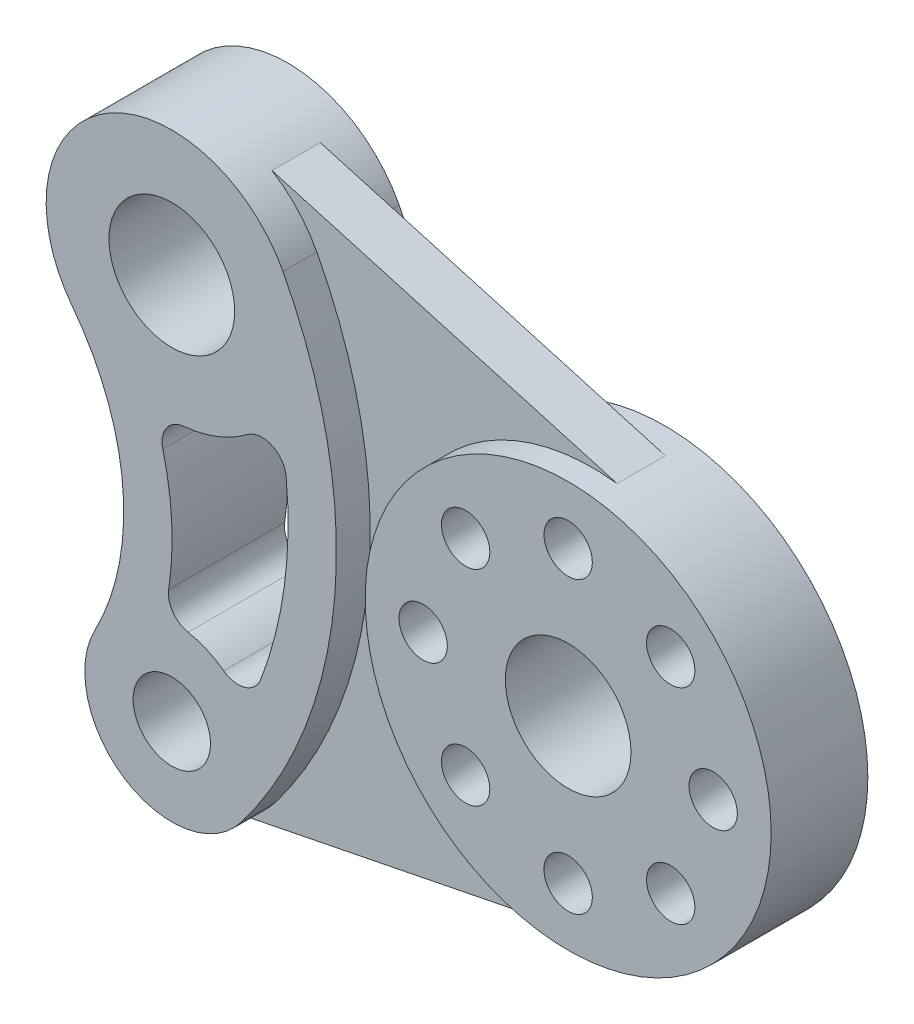
ISO-10303-21;
HEADER;
FILE_DESCRIPTION(('STEP AP214'),'2;1');
FILE_NAME('part.step','',(''),(''),'','','');
FILE_SCHEMA(('AUTOMOTIVE_DESIGN { 1 0 10303 214 1 1 1 1 }'));
ENDSEC;
DATA;
#1=APPLICATION_CONTEXT('core data for automotive mechanical design processes');
#2=APPLICATION_PROTOCOL_DEFINITION('international standard','automotive_design',2000,#1);
#3=PRODUCT_CONTEXT('',#1,'mechanical');
#4=PRODUCT('Part','Part','',(#3));
#5=PRODUCT_RELATED_PRODUCT_CATEGORY('part','',(#4));
#6=PRODUCT_DEFINITION_FORMATION('','',#4);
#7=PRODUCT_DEFINITION_CONTEXT('part definition',#1,'design');
#8=PRODUCT_DEFINITION('design','',#6,#7);
#9=PRODUCT_DEFINITION_SHAPE('','',#8);
#10=(LENGTH_UNIT() NAMED_UNIT(*) SI_UNIT(.MILLI.,.METRE.));
#11=(NAMED_UNIT(*) PLANE_ANGLE_UNIT() SI_UNIT($,.RADIAN.));
#12=(NAMED_UNIT(*) SI_UNIT($,.STERADIAN.) SOLID_ANGLE_UNIT());
#13=UNCERTAINTY_MEASURE_WITH_UNIT(LENGTH_MEASURE(1.E-05),#10,'distance_accuracy_value','');
#14=(GEOMETRIC_REPRESENTATION_CONTEXT(3) GLOBAL_UNCERTAINTY_ASSIGNED_CONTEXT((#13)) GLOBAL_UNIT_ASSIGNED_CONTEXT((#10,
#11,#12)) REPRESENTATION_CONTEXT('',''));
#15=CARTESIAN_POINT('',(0.,0.,0.));
#16=DIRECTION('',(0.,0.,1.));
#17=DIRECTION('',(1.,0.,0.));
#18=AXIS2_PLACEMENT_3D('',#15,#16,#17);
#19=CARTESIAN_POINT('',(-80.,-40.,24.));
#20=DIRECTION('',(0.,0.,-1.));
#21=DIRECTION('',(-1.,0.,0.));
#22=AXIS2_PLACEMENT_3D('',#19,#20,#21);
#23=CYLINDRICAL_SURFACE('',#22,18.);
#24=CARTESIAN_POINT('',(-80.,-40.,17.));
#25=DIRECTION('',(0.,0.,-1.));
#26=DIRECTION('',(-1.,0.,0.));
#27=AXIS2_PLACEMENT_3D('',#24,#25,#26);
#28=CIRCLE('',#27,18.);
#29=CARTESIAN_POINT('',(-65.7048938733706,-50.9384615384615,17.));
#30=VERTEX_POINT('',#29);
#31=CARTESIAN_POINT('',(-73.0769230769233,-56.6153846153847,17.));
#32=VERTEX_POINT('',#31);
#33=EDGE_CURVE('E230',#30,#32,#28,.T.);
#34=ORIENTED_EDGE('',*,*,#33,.F.);
#35=DIRECTION('',(0.,0.,-1.));
#36=VECTOR('',#35,1.);
#37=CARTESIAN_POINT('',(-65.7048938733706,-50.9384615384615,24.));
#38=LINE('',#37,#36);
#39=CARTESIAN_POINT('',(-65.7048938733706,-50.9384615384615,24.));
#40=VERTEX_POINT('',#39);
#41=EDGE_CURVE('E326',#40,#30,#38,.T.);
#42=ORIENTED_EDGE('',*,*,#41,.F.);
#43=CARTESIAN_POINT('',(-80.,-40.,24.));
#44=DIRECTION('',(0.,0.,1.));
#45=DIRECTION('',(1.,0.,0.));
#46=AXIS2_PLACEMENT_3D('',#43,#44,#45);
#47=CIRCLE('',#46,18.);
#48=CARTESIAN_POINT('',(-95.9288325411013,-31.6171428571429,24.));
#49=VERTEX_POINT('',#48);
#50=EDGE_CURVE('E271',#49,#40,#47,.T.);
#51=ORIENTED_EDGE('',*,*,#50,.F.);
#52=DIRECTION('',(0.,0.,-1.));
#53=VECTOR('',#52,1.);
#54=CARTESIAN_POINT('',(-95.9288325411013,-31.6171428571429,24.));
#55=LINE('',#54,#53);
#56=CARTESIAN_POINT('',(-95.9288325411013,-31.6171428571429,0.));
#57=VERTEX_POINT('',#56);
#58=EDGE_CURVE('E335',#49,#57,#55,.T.);
#59=ORIENTED_EDGE('',*,*,#58,.T.);
#60=CARTESIAN_POINT('',(-80.,-40.,0.));
#61=DIRECTION('',(0.,0.,1.));
#62=DIRECTION('',(1.,0.,0.));
#63=AXIS2_PLACEMENT_3D('',#60,#61,#62);
#64=CIRCLE('',#63,18.);
#65=CARTESIAN_POINT('',(-65.7048938733706,-50.9384615384615,0.));
#66=VERTEX_POINT('',#65);
#67=EDGE_CURVE('E312',#57,#66,#64,.T.);
#68=ORIENTED_EDGE('',*,*,#67,.T.);
#69=CARTESIAN_POINT('',(-65.7048938733706,-50.9384615384615,7.));
#70=VERTEX_POINT('',#69);
#71=EDGE_CURVE('E329',#70,#66,#38,.T.);
#72=ORIENTED_EDGE('',*,*,#71,.F.);
#73=CARTESIAN_POINT('',(-80.,-40.,7.));
#74=DIRECTION('',(0.,0.,-1.));
#75=DIRECTION('',(-1.,0.,0.));
#76=AXIS2_PLACEMENT_3D('',#73,#74,#75);
#77=CIRCLE('',#76,18.);
#78=CARTESIAN_POINT('',(-73.0769230769233,-56.6153846153847,7.));
#79=VERTEX_POINT('',#78);
#80=EDGE_CURVE('E217',#70,#79,#77,.T.);
#81=ORIENTED_EDGE('',*,*,#80,.T.);
#82=DIRECTION('',(0.,0.,-1.));
#83=VECTOR('',#82,1.);
#84=CARTESIAN_POINT('',(-73.0769230769233,-56.6153846153847,24.));
#85=LINE('',#84,#83);
#86=EDGE_CURVE('E11',#32,#79,#85,.T.);
#87=ORIENTED_EDGE('',*,*,#86,.F.);
#88=EDGE_LOOP('',(#34,#42,#51,#59,#68,#72,#81,#87));
#89=FACE_BOUND('',#88,.T.);
#90=ADVANCED_FACE('F50',(#89),#23,.T.);
#91=CARTESIAN_POINT('',(-141.945459882061,7.39999999999997,24.));
#92=DIRECTION('',(0.,0.,-1.));
#93=DIRECTION('',(-1.,0.,0.));
#94=AXIS2_PLACEMENT_3D('',#91,#92,#93);
#95=CYLINDRICAL_SURFACE('',#94,96.);
#96=ORIENTED_EDGE('',*,*,#41,.T.);
#97=CARTESIAN_POINT('',(-141.945459882061,7.39999999999997,17.));
#98=DIRECTION('',(0.,0.,-1.));
#99=DIRECTION('',(-1.,0.,0.));
#100=AXIS2_PLACEMENT_3D('',#97,#98,#99);
#101=CIRCLE('',#100,96.);
#102=CARTESIAN_POINT('',(-56.9916863295203,52.1085714285714,17.));
#103=VERTEX_POINT('',#102);
#104=EDGE_CURVE('E228',#30,#103,#101,.F.);
#105=ORIENTED_EDGE('',*,*,#104,.T.);
#106=DIRECTION('',(0.,0.,-1.));
#107=VECTOR('',#106,1.);
#108=CARTESIAN_POINT('',(-56.9916863295203,52.1085714285714,24.));
#109=LINE('',#108,#107);
#110=CARTESIAN_POINT('',(-56.9916863295203,52.1085714285714,24.));
#111=VERTEX_POINT('',#110);
#112=EDGE_CURVE('E323',#111,#103,#109,.T.);
#113=ORIENTED_EDGE('',*,*,#112,.F.);
#114=CARTESIAN_POINT('',(-141.945459882061,7.39999999999997,24.));
#115=DIRECTION('',(0.,0.,1.));
#116=DIRECTION('',(1.,0.,0.));
#117=AXIS2_PLACEMENT_3D('',#114,#115,#116);
#118=CIRCLE('',#117,96.);
#119=EDGE_CURVE('E273',#111,#40,#118,.F.);
#120=ORIENTED_EDGE('',*,*,#119,.T.);
#121=EDGE_LOOP('',(#96,#105,#113,#120));
#122=FACE_BOUND('',#121,.T.);
#123=ADVANCED_FACE('F421',(#122),#95,.T.);
#124=CARTESIAN_POINT('',(-61.3272069104421,15.2547621099623,24.));
#125=DIRECTION('',(0.,0.,-1.));
#126=DIRECTION('',(-1.,0.,0.));
#127=AXIS2_PLACEMENT_3D('',#124,#125,#126);
#128=CYLINDRICAL_SURFACE('',#127,4.99999999999999);
#129=DIRECTION('',(0.,0.,-1.));
#130=VECTOR('',#129,1.);
#131=CARTESIAN_POINT('',(-58.5379091566197,19.4044389697335,12.));
#132=LINE('',#131,#130);
#133=CARTESIAN_POINT('',(-58.5379091566197,19.4044389697336,7.));
#134=VERTEX_POINT('',#133);
#135=CARTESIAN_POINT('',(-58.5379091566197,19.4044389697336,17.));
#136=VERTEX_POINT('',#135);
#137=EDGE_CURVE('E238',#134,#136,#132,.F.);
#138=ORIENTED_EDGE('',*,*,#137,.T.);
#139=CARTESIAN_POINT('',(-61.3272069104421,15.2547621099623,17.));
#140=DIRECTION('',(0.,0.,-1.));
#141=DIRECTION('',(-1.,0.,0.));
#142=AXIS2_PLACEMENT_3D('',#139,#140,#141);
#143=CIRCLE('',#142,4.99999999999999);
#144=CARTESIAN_POINT('',(-56.3507715418237,15.7396239686019,17.));
#145=VERTEX_POINT('',#144);
#146=EDGE_CURVE('E231',#136,#145,#143,.T.);
#147=ORIENTED_EDGE('',*,*,#146,.T.);
#148=DIRECTION('',(0.,0.,-1.));
#149=VECTOR('',#148,1.);
#150=CARTESIAN_POINT('',(-56.3507715418237,15.7396239686019,24.));
#151=LINE('',#150,#149);
#152=CARTESIAN_POINT('',(-56.3507715418237,15.7396239686019,24.));
#153=VERTEX_POINT('',#152);
#154=EDGE_CURVE('E347',#153,#145,#151,.T.);
#155=ORIENTED_EDGE('',*,*,#154,.F.);
#156=CARTESIAN_POINT('',(-61.3272069104421,15.2547621099623,24.));
#157=DIRECTION('',(0.,0.,1.));
#158=DIRECTION('',(1.,0.,0.));
#159=AXIS2_PLACEMENT_3D('',#156,#157,#158);
#160=CIRCLE('',#159,4.99999999999999);
#161=CARTESIAN_POINT('',(-64.3389477313385,19.2459295115812,24.));
#162=VERTEX_POINT('',#161);
#163=EDGE_CURVE('E247',#153,#162,#160,.T.);
#164=ORIENTED_EDGE('',*,*,#163,.T.);
#165=DIRECTION('',(0.,0.,-1.));
#166=VECTOR('',#165,1.);
#167=CARTESIAN_POINT('',(-64.3389477313385,19.2459295115812,24.));
#168=LINE('',#167,#166);
#169=CARTESIAN_POINT('',(-64.3389477313385,19.2459295115812,0.));
#170=VERTEX_POINT('',#169);
#171=EDGE_CURVE('E346',#162,#170,#168,.T.);
#172=ORIENTED_EDGE('',*,*,#171,.T.);
#173=CARTESIAN_POINT('',(-61.3272069104421,15.2547621099623,0.));
#174=DIRECTION('',(0.,0.,1.));
#175=DIRECTION('',(1.,0.,0.));
#176=AXIS2_PLACEMENT_3D('',#173,#174,#175);
#177=CIRCLE('',#176,4.99999999999999);
#178=CARTESIAN_POINT('',(-56.3507715418237,15.7396239686019,0.));
#179=VERTEX_POINT('',#178);
#180=EDGE_CURVE('E286',#179,#170,#177,.T.);
#181=ORIENTED_EDGE('',*,*,#180,.F.);
#182=CARTESIAN_POINT('',(-56.3507715418237,15.7396239686019,7.));
#183=VERTEX_POINT('',#182);
#184=EDGE_CURVE('E343',#183,#179,#151,.T.);
#185=ORIENTED_EDGE('',*,*,#184,.F.);
#186=CARTESIAN_POINT('',(-61.3272069104421,15.2547621099623,7.));
#187=DIRECTION('',(0.,0.,-1.));
#188=DIRECTION('',(-1.,0.,0.));
#189=AXIS2_PLACEMENT_3D('',#186,#187,#188);
#190=CIRCLE('',#189,4.99999999999999);
#191=EDGE_CURVE('E61',#134,#183,#190,.T.);
#192=ORIENTED_EDGE('',*,*,#191,.F.);
#193=EDGE_LOOP('',(#138,#147,#155,#164,#172,#181,#185,#192));
#194=FACE_BOUND('',#193,.T.);
#195=ADVANCED_FACE('F462',(#194),#128,.F.);
#196=CARTESIAN_POINT('',(-141.945459882061,7.39999999999997,24.));
#197=DIRECTION('',(0.,0.,-1.));
#198=DIRECTION('',(-1.,0.,0.));
#199=AXIS2_PLACEMENT_3D('',#196,#197,#198);
#200=CYLINDRICAL_SURFACE('',#199,86.);
#201=CARTESIAN_POINT('',(-141.945459882061,7.39999999999997,17.));
#202=DIRECTION('',(0.,0.,-1.));
#203=DIRECTION('',(-1.,0.,0.));
#204=AXIS2_PLACEMENT_3D('',#201,#202,#203);
#205=CIRCLE('',#204,86.);
#206=CARTESIAN_POINT('',(-60.0640049531022,-18.8950059653334,17.));
#207=VERTEX_POINT('',#206);
#208=EDGE_CURVE('E233',#207,#145,#205,.F.);
#209=ORIENTED_EDGE('',*,*,#208,.F.);
#210=DIRECTION('',(0.,0.,-1.));
#211=VECTOR('',#210,1.);
#212=CARTESIAN_POINT('',(-60.0640049531022,-18.8950059653334,12.));
#213=LINE('',#212,#211);
#214=CARTESIAN_POINT('',(-60.0640049531022,-18.8950059653334,6.99999999999999));
#215=VERTEX_POINT('',#214);
#216=EDGE_CURVE('E236',#215,#207,#213,.F.);
#217=ORIENTED_EDGE('',*,*,#216,.F.);
#218=CARTESIAN_POINT('',(-141.945459882061,7.39999999999997,7.));
#219=DIRECTION('',(0.,0.,-1.));
#220=DIRECTION('',(-1.,0.,0.));
#221=AXIS2_PLACEMENT_3D('',#218,#219,#220);
#222=CIRCLE('',#221,86.);
#223=EDGE_CURVE('E223',#215,#183,#222,.F.);
#224=ORIENTED_EDGE('',*,*,#223,.T.);
#225=ORIENTED_EDGE('',*,*,#184,.T.);
#226=CARTESIAN_POINT('',(-141.945459882061,7.39999999999997,0.));
#227=DIRECTION('',(0.,0.,1.));
#228=DIRECTION('',(1.,0.,0.));
#229=AXIS2_PLACEMENT_3D('',#226,#227,#228);
#230=CIRCLE('',#229,86.);
#231=CARTESIAN_POINT('',(-61.6191338065602,-23.319396791154,0.));
#232=VERTEX_POINT('',#231);
#233=EDGE_CURVE('E287',#179,#232,#230,.F.);
#234=ORIENTED_EDGE('',*,*,#233,.T.);
#235=DIRECTION('',(0.,0.,-1.));
#236=VECTOR('',#235,1.);
#237=CARTESIAN_POINT('',(-61.6191338065602,-23.319396791154,24.));
#238=LINE('',#237,#236);
#239=CARTESIAN_POINT('',(-61.6191338065602,-23.319396791154,24.));
#240=VERTEX_POINT('',#239);
#241=EDGE_CURVE('E344',#240,#232,#238,.T.);
#242=ORIENTED_EDGE('',*,*,#241,.F.);
#243=CARTESIAN_POINT('',(-141.945459882061,7.39999999999997,24.));
#244=DIRECTION('',(0.,0.,1.));
#245=DIRECTION('',(1.,0.,0.));
#246=AXIS2_PLACEMENT_3D('',#243,#244,#245);
#247=CIRCLE('',#246,86.);
#248=EDGE_CURVE('E252',#153,#240,#247,.F.);
#249=ORIENTED_EDGE('',*,*,#248,.F.);
#250=ORIENTED_EDGE('',*,*,#154,.T.);
#251=EDGE_LOOP('',(#209,#217,#224,#225,#234,#242,#249,#250));
#252=FACE_BOUND('',#251,.T.);
#253=ADVANCED_FACE('F490',(#252),#200,.F.);
#254=CARTESIAN_POINT('',(-80.,40.,24.));
#255=DIRECTION('',(0.,0.,-1.));
#256=DIRECTION('',(-1.,0.,0.));
#257=AXIS2_PLACEMENT_3D('',#254,#255,#256);
#258=CYLINDRICAL_SURFACE('',#257,26.);
#259=CARTESIAN_POINT('',(-80.,40.,17.));
#260=DIRECTION('',(0.,0.,-1.));
#261=DIRECTION('',(-1.,0.,0.));
#262=AXIS2_PLACEMENT_3D('',#259,#260,#261);
#263=CIRCLE('',#262,26.);
#264=CARTESIAN_POINT('',(-66.2671037182628,62.0773087063403,17.));
#265=VERTEX_POINT('',#264);
#266=EDGE_CURVE('E57',#265,#103,#263,.T.);
#267=ORIENTED_EDGE('',*,*,#266,.F.);
#268=DIRECTION('',(0.,0.,-1.));
#269=VECTOR('',#268,1.);
#270=CARTESIAN_POINT('',(-66.2671037182628,62.0773087063403,24.));
#271=LINE('',#270,#269);
#272=CARTESIAN_POINT('',(-66.2671037182628,62.0773087063403,7.));
#273=VERTEX_POINT('',#272);
#274=EDGE_CURVE('E353',#273,#265,#271,.F.);
#275=ORIENTED_EDGE('',*,*,#274,.F.);
#276=CARTESIAN_POINT('',(-80.,40.,7.));
#277=DIRECTION('',(0.,0.,-1.));
#278=DIRECTION('',(-1.,0.,0.));
#279=AXIS2_PLACEMENT_3D('',#276,#277,#278);
#280=CIRCLE('',#279,26.);
#281=CARTESIAN_POINT('',(-56.9916863295203,52.1085714285714,7.));
#282=VERTEX_POINT('',#281);
#283=EDGE_CURVE('E334',#273,#282,#280,.T.);
#284=ORIENTED_EDGE('',*,*,#283,.T.);
#285=CARTESIAN_POINT('',(-56.9916863295203,52.1085714285714,0.));
#286=VERTEX_POINT('',#285);
#287=EDGE_CURVE('E324',#282,#286,#109,.T.);
#288=ORIENTED_EDGE('',*,*,#287,.T.);
#289=CARTESIAN_POINT('',(-80.,40.,0.));
#290=DIRECTION('',(0.,0.,1.));
#291=DIRECTION('',(1.,0.,0.));
#292=AXIS2_PLACEMENT_3D('',#289,#290,#291);
#293=CIRCLE('',#292,26.);
#294=CARTESIAN_POINT('',(-100.648486627354,24.2,0.));
#295=VERTEX_POINT('',#294);
#296=EDGE_CURVE('E246',#286,#295,#293,.T.);
#297=ORIENTED_EDGE('',*,*,#296,.T.);
#298=DIRECTION('',(0.,0.,-1.));
#299=VECTOR('',#298,1.);
#300=CARTESIAN_POINT('',(-100.648486627354,24.2,24.));
#301=LINE('',#300,#299);
#302=CARTESIAN_POINT('',(-100.648486627354,24.2,24.));
#303=VERTEX_POINT('',#302);
#304=EDGE_CURVE('E318',#303,#295,#301,.T.);
#305=ORIENTED_EDGE('',*,*,#304,.F.);
#306=CARTESIAN_POINT('',(-80.,40.,24.));
#307=DIRECTION('',(0.,0.,1.));
#308=DIRECTION('',(1.,0.,0.));
#309=AXIS2_PLACEMENT_3D('',#306,#307,#308);
#310=CIRCLE('',#309,26.);
#311=EDGE_CURVE('E279',#111,#303,#310,.T.);
#312=ORIENTED_EDGE('',*,*,#311,.F.);
#313=ORIENTED_EDGE('',*,*,#112,.T.);
#314=EDGE_LOOP('',(#267,#275,#284,#288,#297,#305,#312,#313));
#315=FACE_BOUND('',#314,.T.);
#316=ADVANCED_FACE('F416',(#315),#258,.T.);
#317=CARTESIAN_POINT('',(-141.945459882061,-7.40000000000002,24.));
#318=DIRECTION('',(0.,0.,-1.));
#319=DIRECTION('',(-1.,0.,0.));
#320=AXIS2_PLACEMENT_3D('',#317,#318,#319);
#321=CYLINDRICAL_SURFACE('',#320,52.);
#322=CARTESIAN_POINT('',(-141.945459882061,-7.40000000000002,0.));
#323=DIRECTION('',(0.,0.,1.));
#324=DIRECTION('',(1.,0.,0.));
#325=AXIS2_PLACEMENT_3D('',#322,#323,#324);
#326=CIRCLE('',#325,52.);
#327=EDGE_CURVE('E309',#295,#57,#326,.F.);
#328=ORIENTED_EDGE('',*,*,#327,.T.);
#329=ORIENTED_EDGE('',*,*,#58,.F.);
#330=CARTESIAN_POINT('',(-141.945459882061,-7.40000000000002,24.));
#331=DIRECTION('',(0.,0.,1.));
#332=DIRECTION('',(1.,0.,0.));
#333=AXIS2_PLACEMENT_3D('',#330,#331,#332);
#334=CIRCLE('',#333,52.);
#335=EDGE_CURVE('E269',#303,#49,#334,.F.);
#336=ORIENTED_EDGE('',*,*,#335,.F.);
#337=ORIENTED_EDGE('',*,*,#304,.T.);
#338=EDGE_LOOP('',(#328,#329,#336,#337));
#339=FACE_BOUND('',#338,.T.);
#340=ADVANCED_FACE('F438',(#339),#321,.F.);
#341=CARTESIAN_POINT('',(-141.945459882061,7.39999999999997,7.));
#342=DIRECTION('',(0.,0.,-1.));
#343=DIRECTION('',(-1.,0.,0.));
#344=AXIS2_PLACEMENT_3D('',#341,#342,#343);
#345=CIRCLE('',#344,96.);
#346=EDGE_CURVE('E75',#70,#282,#345,.F.);
#347=ORIENTED_EDGE('',*,*,#346,.F.);
#348=ORIENTED_EDGE('',*,*,#71,.T.);
#349=CARTESIAN_POINT('',(-141.945459882061,7.39999999999997,0.));
#350=DIRECTION('',(0.,0.,1.));
#351=DIRECTION('',(1.,0.,0.));
#352=AXIS2_PLACEMENT_3D('',#349,#350,#351);
#353=CIRCLE('',#352,96.);
#354=EDGE_CURVE('E317',#286,#66,#353,.F.);
#355=ORIENTED_EDGE('',*,*,#354,.F.);
#356=ORIENTED_EDGE('',*,*,#287,.F.);
#357=EDGE_LOOP('',(#347,#348,#355,#356));
#358=FACE_BOUND('',#357,.T.);
#359=ADVANCED_FACE('F429',(#358),#95,.T.);
#360=CARTESIAN_POINT('',(-77.0200366306394,9.1435611530224,24.));
#361=DIRECTION('',(0.,0.,-1.));
#362=DIRECTION('',(-1.,0.,0.));
#363=AXIS2_PLACEMENT_3D('',#360,#361,#362);
#364=CYLINDRICAL_SURFACE('',#363,4.99999999999999);
#365=CARTESIAN_POINT('',(-77.0200366306394,9.1435611530224,0.));
#366=DIRECTION('',(0.,0.,1.));
#367=DIRECTION('',(1.,0.,0.));
#368=AXIS2_PLACEMENT_3D('',#365,#366,#367);
#369=CIRCLE('',#368,4.99999999999999);
#370=CARTESIAN_POINT('',(-77.5006758837621,14.1204061283414,0.));
#371=VERTEX_POINT('',#370);
#372=CARTESIAN_POINT('',(-81.8652174702977,7.90896703712521,0.));
#373=VERTEX_POINT('',#372);
#374=EDGE_CURVE('E241',#371,#373,#369,.T.);
#375=ORIENTED_EDGE('',*,*,#374,.F.);
#376=DIRECTION('',(0.,0.,-1.));
#377=VECTOR('',#376,1.);
#378=CARTESIAN_POINT('',(-77.5006758837621,14.1204061283414,24.));
#379=LINE('',#378,#377);
#380=CARTESIAN_POINT('',(-77.5006758837621,14.1204061283414,24.));
#381=VERTEX_POINT('',#380);
#382=EDGE_CURVE('E321',#381,#371,#379,.T.);
#383=ORIENTED_EDGE('',*,*,#382,.F.);
#384=CARTESIAN_POINT('',(-77.0200366306394,9.1435611530224,24.));
#385=DIRECTION('',(0.,0.,1.));
#386=DIRECTION('',(1.,0.,0.));
#387=AXIS2_PLACEMENT_3D('',#384,#385,#386);
#388=CIRCLE('',#387,4.99999999999999);
#389=CARTESIAN_POINT('',(-81.8652174702977,7.90896703712521,24.));
#390=VERTEX_POINT('',#389);
#391=EDGE_CURVE('E245',#381,#390,#388,.T.);
#392=ORIENTED_EDGE('',*,*,#391,.T.);
#393=DIRECTION('',(0.,0.,-1.));
#394=VECTOR('',#393,1.);
#395=CARTESIAN_POINT('',(-81.8652174702977,7.90896703712521,24.));
#396=LINE('',#395,#394);
#397=EDGE_CURVE('E278',#390,#373,#396,.T.);
#398=ORIENTED_EDGE('',*,*,#397,.T.);
#399=EDGE_LOOP('',(#375,#383,#392,#398));
#400=FACE_BOUND('',#399,.T.);
#401=ADVANCED_FACE('F47',(#400),#364,.F.);
#402=CARTESIAN_POINT('',(-80.,40.,24.));
#403=DIRECTION('',(0.,0.,-1.));
#404=DIRECTION('',(-1.,0.,0.));
#405=AXIS2_PLACEMENT_3D('',#402,#403,#404);
#406=CYLINDRICAL_SURFACE('',#405,26.);
#407=CARTESIAN_POINT('',(-80.,40.,0.));
#408=DIRECTION('',(0.,0.,1.));
#409=DIRECTION('',(1.,0.,0.));
#410=AXIS2_PLACEMENT_3D('',#407,#408,#409);
#411=CIRCLE('',#410,26.);
#412=EDGE_CURVE('E284',#371,#170,#411,.T.);
#413=ORIENTED_EDGE('',*,*,#412,.T.);
#414=ORIENTED_EDGE('',*,*,#171,.F.);
#415=CARTESIAN_POINT('',(-80.,40.,24.));
#416=DIRECTION('',(0.,0.,1.));
#417=DIRECTION('',(1.,0.,0.));
#418=AXIS2_PLACEMENT_3D('',#415,#416,#417);
#419=CIRCLE('',#418,26.);
#420=EDGE_CURVE('E244',#381,#162,#419,.T.);
#421=ORIENTED_EDGE('',*,*,#420,.F.);
#422=ORIENTED_EDGE('',*,*,#382,.T.);
#423=EDGE_LOOP('',(#413,#414,#421,#422));
#424=FACE_BOUND('',#423,.T.);
#425=ADVANCED_FACE('F487',(#424),#406,.T.);
#426=CARTESIAN_POINT('',(-66.2892690435079,-21.5333853498079,24.));
#427=DIRECTION('',(0.,0.,-1.));
#428=DIRECTION('',(-1.,0.,0.));
#429=AXIS2_PLACEMENT_3D('',#426,#427,#428);
#430=CYLINDRICAL_SURFACE('',#429,4.99999999999999);
#431=CARTESIAN_POINT('',(-66.2892690435079,-21.5333853498079,0.));
#432=DIRECTION('',(0.,0.,1.));
#433=DIRECTION('',(1.,0.,0.));
#434=AXIS2_PLACEMENT_3D('',#431,#432,#433);
#435=CIRCLE('',#434,4.99999999999999);
#436=CARTESIAN_POINT('',(-69.2698627297019,-25.5478667955018,0.));
#437=VERTEX_POINT('',#436);
#438=EDGE_CURVE('E292',#437,#232,#435,.T.);
#439=ORIENTED_EDGE('',*,*,#438,.F.);
#440=DIRECTION('',(0.,0.,-1.));
#441=VECTOR('',#440,1.);
#442=CARTESIAN_POINT('',(-69.2698627297019,-25.5478667955018,24.));
#443=LINE('',#442,#441);
#444=CARTESIAN_POINT('',(-69.2698627297019,-25.5478667955018,24.));
#445=VERTEX_POINT('',#444);
#446=EDGE_CURVE('E342',#445,#437,#443,.T.);
#447=ORIENTED_EDGE('',*,*,#446,.F.);
#448=CARTESIAN_POINT('',(-66.2892690435079,-21.5333853498079,24.));
#449=DIRECTION('',(0.,0.,1.));
#450=DIRECTION('',(1.,0.,0.));
#451=AXIS2_PLACEMENT_3D('',#448,#449,#450);
#452=CIRCLE('',#451,4.99999999999999);
#453=EDGE_CURVE('E254',#445,#240,#452,.T.);
#454=ORIENTED_EDGE('',*,*,#453,.T.);
#455=ORIENTED_EDGE('',*,*,#241,.T.);
#456=EDGE_LOOP('',(#439,#447,#454,#455));
#457=FACE_BOUND('',#456,.T.);
#458=ADVANCED_FACE('F483',(#457),#430,.F.);
#459=CARTESIAN_POINT('',(-80.,-40.,24.));
#460=DIRECTION('',(0.,0.,-1.));
#461=DIRECTION('',(-1.,0.,0.));
#462=AXIS2_PLACEMENT_3D('',#459,#460,#461);
#463=CYLINDRICAL_SURFACE('',#462,18.);
#464=CARTESIAN_POINT('',(-80.,-40.,0.));
#465=DIRECTION('',(0.,0.,1.));
#466=DIRECTION('',(1.,0.,0.));
#467=AXIS2_PLACEMENT_3D('',#464,#465,#466);
#468=CIRCLE('',#467,18.);
#469=CARTESIAN_POINT('',(-76.632322995635,-22.3178408672959,0.));
#470=VERTEX_POINT('',#469);
#471=EDGE_CURVE('E294',#437,#470,#468,.T.);
#472=ORIENTED_EDGE('',*,*,#471,.T.);
#473=DIRECTION('',(0.,0.,-1.));
#474=VECTOR('',#473,1.);
#475=CARTESIAN_POINT('',(-76.632322995635,-22.3178408672959,24.));
#476=LINE('',#475,#474);
#477=CARTESIAN_POINT('',(-76.632322995635,-22.3178408672959,24.));
#478=VERTEX_POINT('',#477);
#479=EDGE_CURVE('E339',#478,#470,#476,.T.);
#480=ORIENTED_EDGE('',*,*,#479,.F.);
#481=CARTESIAN_POINT('',(-80.,-40.,24.));
#482=DIRECTION('',(0.,0.,1.));
#483=DIRECTION('',(1.,0.,0.));
#484=AXIS2_PLACEMENT_3D('',#481,#482,#483);
#485=CIRCLE('',#484,18.);
#486=EDGE_CURVE('E257',#445,#478,#485,.T.);
#487=ORIENTED_EDGE('',*,*,#486,.F.);
#488=ORIENTED_EDGE('',*,*,#446,.T.);
#489=EDGE_LOOP('',(#472,#480,#487,#488));
#490=FACE_BOUND('',#489,.T.);
#491=ADVANCED_FACE('F476',(#490),#463,.T.);
#492=CARTESIAN_POINT('',(-75.6968571610891,-17.4061299971003,24.));
#493=DIRECTION('',(0.,0.,-1.));
#494=DIRECTION('',(-1.,0.,0.));
#495=AXIS2_PLACEMENT_3D('',#492,#493,#494);
#496=CYLINDRICAL_SURFACE('',#495,5.);
#497=CARTESIAN_POINT('',(-75.6968571610891,-17.4061299971003,0.));
#498=DIRECTION('',(0.,0.,1.));
#499=DIRECTION('',(1.,0.,0.));
#500=AXIS2_PLACEMENT_3D('',#497,#498,#499);
#501=CIRCLE('',#500,5.);
#502=CARTESIAN_POINT('',(-80.640782737281,-16.6594038779137,0.));
#503=VERTEX_POINT('',#502);
#504=EDGE_CURVE('E296',#503,#470,#501,.T.);
#505=ORIENTED_EDGE('',*,*,#504,.F.);
#506=DIRECTION('',(0.,0.,-1.));
#507=VECTOR('',#506,1.);
#508=CARTESIAN_POINT('',(-80.640782737281,-16.6594038779137,24.));
#509=LINE('',#508,#507);
#510=CARTESIAN_POINT('',(-80.640782737281,-16.6594038779137,24.));
#511=VERTEX_POINT('',#510);
#512=EDGE_CURVE('E340',#511,#503,#509,.T.);
#513=ORIENTED_EDGE('',*,*,#512,.F.);
#514=CARTESIAN_POINT('',(-75.6968571610891,-17.4061299971003,24.));
#515=DIRECTION('',(0.,0.,1.));
#516=DIRECTION('',(1.,0.,0.));
#517=AXIS2_PLACEMENT_3D('',#514,#515,#516);
#518=CIRCLE('',#517,5.);
#519=EDGE_CURVE('E259',#511,#478,#518,.T.);
#520=ORIENTED_EDGE('',*,*,#519,.T.);
#521=ORIENTED_EDGE('',*,*,#479,.T.);
#522=EDGE_LOOP('',(#505,#513,#520,#521));
#523=FACE_BOUND('',#522,.T.);
#524=ADVANCED_FACE('F475',(#523),#496,.F.);
#525=CARTESIAN_POINT('',(-80.,-40.,24.));
#526=DIRECTION('',(0.,0.,-1.));
#527=DIRECTION('',(-1.,0.,0.));
#528=AXIS2_PLACEMENT_3D('',#525,#526,#527);
#529=CYLINDRICAL_SURFACE('',#528,8.);
#530=CARTESIAN_POINT('',(-80.,-40.,24.));
#531=DIRECTION('',(0.,0.,1.));
#532=DIRECTION('',(1.,0.,0.));
#533=AXIS2_PLACEMENT_3D('',#530,#531,#532);
#534=CIRCLE('',#533,8.);
#535=CARTESIAN_POINT('',(-72.,-40.,24.));
#536=VERTEX_POINT('',#535);
#537=EDGE_CURVE('E270',#536,#536,#534,.T.);
#538=ORIENTED_EDGE('',*,*,#537,.T.);
#539=EDGE_LOOP('',(#538));
#540=FACE_BOUND('',#539,.T.);
#541=CARTESIAN_POINT('',(-80.,-40.,0.));
#542=DIRECTION('',(0.,0.,1.));
#543=DIRECTION('',(1.,0.,0.));
#544=AXIS2_PLACEMENT_3D('',#541,#542,#543);
#545=CIRCLE('',#544,8.);
#546=CARTESIAN_POINT('',(-72.,-40.,0.));
#547=VERTEX_POINT('',#546);
#548=EDGE_CURVE('E310',#547,#547,#545,.T.);
#549=ORIENTED_EDGE('',*,*,#548,.F.);
#550=EDGE_LOOP('',(#549));
#551=FACE_BOUND('',#550,.T.);
#552=ADVANCED_FACE('F469',(#540,#551),#529,.F.);
#553=CARTESIAN_POINT('',(-80.,40.,24.));
#554=DIRECTION('',(0.,0.,-1.));
#555=DIRECTION('',(-1.,0.,0.));
#556=AXIS2_PLACEMENT_3D('',#553,#554,#555);
#557=CYLINDRICAL_SURFACE('',#556,13.);
#558=CARTESIAN_POINT('',(-80.,40.,24.));
#559=DIRECTION('',(0.,0.,1.));
#560=DIRECTION('',(1.,0.,0.));
#561=AXIS2_PLACEMENT_3D('',#558,#559,#560);
#562=CIRCLE('',#561,13.);
#563=CARTESIAN_POINT('',(-67.,40.,24.));
#564=VERTEX_POINT('',#563);
#565=EDGE_CURVE('E261',#564,#564,#562,.T.);
#566=ORIENTED_EDGE('',*,*,#565,.T.);
#567=EDGE_LOOP('',(#566));
#568=FACE_BOUND('',#567,.T.);
#569=CARTESIAN_POINT('',(-80.,40.,0.));
#570=DIRECTION('',(0.,0.,1.));
#571=DIRECTION('',(1.,0.,0.));
#572=AXIS2_PLACEMENT_3D('',#569,#570,#571);
#573=CIRCLE('',#572,13.);
#574=CARTESIAN_POINT('',(-67.,40.,0.));
#575=VERTEX_POINT('',#574);
#576=EDGE_CURVE('E302',#575,#575,#573,.T.);
#577=ORIENTED_EDGE('',*,*,#576,.F.);
#578=EDGE_LOOP('',(#577));
#579=FACE_BOUND('',#578,.T.);
#580=ADVANCED_FACE('F454',(#568,#579),#557,.F.);
#581=CARTESIAN_POINT('',(-141.945459882061,-7.40000000000002,24.));
#582=DIRECTION('',(0.,0.,-1.));
#583=DIRECTION('',(-1.,0.,0.));
#584=AXIS2_PLACEMENT_3D('',#581,#582,#583);
#585=CYLINDRICAL_SURFACE('',#584,62.);
#586=CARTESIAN_POINT('',(-141.945459882061,-7.40000000000002,0.));
#587=DIRECTION('',(0.,0.,1.));
#588=DIRECTION('',(1.,0.,0.));
#589=AXIS2_PLACEMENT_3D('',#586,#587,#588);
#590=CIRCLE('',#589,62.);
#591=EDGE_CURVE('E301',#373,#503,#590,.F.);
#592=ORIENTED_EDGE('',*,*,#591,.F.);
#593=ORIENTED_EDGE('',*,*,#397,.F.);
#594=CARTESIAN_POINT('',(-141.945459882061,-7.40000000000002,24.));
#595=DIRECTION('',(0.,0.,1.));
#596=DIRECTION('',(1.,0.,0.));
#597=AXIS2_PLACEMENT_3D('',#594,#595,#596);
#598=CIRCLE('',#597,62.);
#599=EDGE_CURVE('E262',#390,#511,#598,.F.);
#600=ORIENTED_EDGE('',*,*,#599,.T.);
#601=ORIENTED_EDGE('',*,*,#512,.T.);
#602=EDGE_LOOP('',(#592,#593,#600,#601));
#603=FACE_BOUND('',#602,.T.);
#604=ADVANCED_FACE('F442',(#603),#585,.T.);
#605=CARTESIAN_POINT('',(0.,0.,24.));
#606=DIRECTION('',(0.,0.,1.));
#607=DIRECTION('',(1.,0.,0.));
#608=AXIS2_PLACEMENT_3D('',#605,#606,#607);
#609=PLANE('',#608);
#610=ORIENTED_EDGE('',*,*,#391,.F.);
#611=ORIENTED_EDGE('',*,*,#420,.T.);
#612=ORIENTED_EDGE('',*,*,#163,.F.);
#613=ORIENTED_EDGE('',*,*,#248,.T.);
#614=ORIENTED_EDGE('',*,*,#453,.F.);
#615=ORIENTED_EDGE('',*,*,#486,.T.);
#616=ORIENTED_EDGE('',*,*,#519,.F.);
#617=ORIENTED_EDGE('',*,*,#599,.F.);
#618=EDGE_LOOP('',(#610,#611,#612,#613,#614,#615,#616,#617));
#619=FACE_BOUND('',#618,.T.);
#620=ORIENTED_EDGE('',*,*,#565,.F.);
#621=EDGE_LOOP('',(#620));
#622=FACE_BOUND('',#621,.T.);
#623=ORIENTED_EDGE('',*,*,#537,.F.);
#624=EDGE_LOOP('',(#623));
#625=FACE_BOUND('',#624,.T.);
#626=ORIENTED_EDGE('',*,*,#335,.T.);
#627=ORIENTED_EDGE('',*,*,#50,.T.);
#628=ORIENTED_EDGE('',*,*,#119,.F.);
#629=ORIENTED_EDGE('',*,*,#311,.T.);
#630=EDGE_LOOP('',(#626,#627,#628,#629));
#631=FACE_BOUND('',#630,.T.);
#632=ADVANCED_FACE('F441',(#619,#622,#625,#631),#609,.T.);
#633=CARTESIAN_POINT('',(0.,0.,0.));
#634=DIRECTION('',(0.,0.,1.));
#635=DIRECTION('',(1.,0.,0.));
#636=AXIS2_PLACEMENT_3D('',#633,#634,#635);
#637=PLANE('',#636);
#638=ORIENTED_EDGE('',*,*,#374,.T.);
#639=ORIENTED_EDGE('',*,*,#591,.T.);
#640=ORIENTED_EDGE('',*,*,#504,.T.);
#641=ORIENTED_EDGE('',*,*,#471,.F.);
#642=ORIENTED_EDGE('',*,*,#438,.T.);
#643=ORIENTED_EDGE('',*,*,#233,.F.);
#644=ORIENTED_EDGE('',*,*,#180,.T.);
#645=ORIENTED_EDGE('',*,*,#412,.F.);
#646=EDGE_LOOP('',(#638,#639,#640,#641,#642,#643,#644,#645));
#647=FACE_BOUND('',#646,.T.);
#648=ORIENTED_EDGE('',*,*,#576,.T.);
#649=EDGE_LOOP('',(#648));
#650=FACE_BOUND('',#649,.T.);
#651=ORIENTED_EDGE('',*,*,#548,.T.);
#652=EDGE_LOOP('',(#651));
#653=FACE_BOUND('',#652,.T.);
#654=ORIENTED_EDGE('',*,*,#327,.F.);
#655=ORIENTED_EDGE('',*,*,#296,.F.);
#656=ORIENTED_EDGE('',*,*,#354,.T.);
#657=ORIENTED_EDGE('',*,*,#67,.F.);
#658=EDGE_LOOP('',(#654,#655,#656,#657));
#659=FACE_BOUND('',#658,.T.);
#660=ADVANCED_FACE('F434',(#647,#650,#653,#659),#637,.F.);
#661=CARTESIAN_POINT('',(-153.293928807235,3.99999999999982,7.));
#662=DIRECTION('',(0.,0.,-1.));
#663=DIRECTION('',(-1.,0.,0.));
#664=AXIS2_PLACEMENT_3D('',#661,#662,#663);
#665=PLANE('',#664);
#666=ORIENTED_EDGE('',*,*,#80,.F.);
#667=ORIENTED_EDGE('',*,*,#346,.T.);
#668=ORIENTED_EDGE('',*,*,#283,.F.);
#669=DIRECTION('',(-0.961542317824901,0.274656824113141,0.));
#670=VECTOR('',#669,1.);
#671=CARTESIAN_POINT('',(-80.0000000000001,66.,7.));
#672=LINE('',#671,#670);
#673=CARTESIAN_POINT('',(5.11632457064738,41.6872069451503,7.));
#674=VERTEX_POINT('',#673);
#675=EDGE_CURVE('E199',#674,#273,#672,.T.);
#676=ORIENTED_EDGE('',*,*,#675,.F.);
#677=CARTESIAN_POINT('',(0.,0.,7.));
#678=DIRECTION('',(0.,0.,-1.));
#679=DIRECTION('',(1.,0.,0.));
#680=AXIS2_PLACEMENT_3D('',#677,#678,#679);
#681=CIRCLE('',#680,42.);
#682=CARTESIAN_POINT('',(0.,-42.,7.));
#683=VERTEX_POINT('',#682);
#684=EDGE_CURVE('E195',#683,#674,#681,.T.);
#685=ORIENTED_EDGE('',*,*,#684,.F.);
#686=DIRECTION('',(0.98058067569092,0.196116135138185,0.));
#687=VECTOR('',#686,1.);
#688=CARTESIAN_POINT('',(0.,-42.,7.));
#689=LINE('',#688,#687);
#690=EDGE_CURVE('E193',#79,#683,#689,.T.);
#691=ORIENTED_EDGE('',*,*,#690,.F.);
#692=EDGE_LOOP('',(#666,#667,#668,#676,#685,#691));
#693=FACE_BOUND('',#692,.T.);
#694=ADVANCED_FACE('F191',(#693),#665,.T.);
#695=CARTESIAN_POINT('',(-153.293928807235,3.99999999999982,17.));
#696=DIRECTION('',(0.,0.,-1.));
#697=DIRECTION('',(-1.,0.,0.));
#698=AXIS2_PLACEMENT_3D('',#695,#696,#697);
#699=PLANE('',#698);
#700=ORIENTED_EDGE('',*,*,#104,.F.);
#701=ORIENTED_EDGE('',*,*,#33,.T.);
#702=DIRECTION('',(0.98058067569092,0.196116135138185,0.));
#703=VECTOR('',#702,1.);
#704=CARTESIAN_POINT('',(0.,-42.,17.));
#705=LINE('',#704,#703);
#706=CARTESIAN_POINT('',(0.,-42.,17.));
#707=VERTEX_POINT('',#706);
#708=EDGE_CURVE('E404',#32,#707,#705,.T.);
#709=ORIENTED_EDGE('',*,*,#708,.T.);
#710=CARTESIAN_POINT('',(0.,0.,17.));
#711=DIRECTION('',(0.,0.,-1.));
#712=DIRECTION('',(1.,0.,0.));
#713=AXIS2_PLACEMENT_3D('',#710,#711,#712);
#714=CIRCLE('',#713,42.);
#715=CARTESIAN_POINT('',(5.11632457064738,41.6872069451503,17.));
#716=VERTEX_POINT('',#715);
#717=EDGE_CURVE('E214',#707,#716,#714,.T.);
#718=ORIENTED_EDGE('',*,*,#717,.T.);
#719=DIRECTION('',(-0.961542317824901,0.274656824113141,0.));
#720=VECTOR('',#719,1.);
#721=CARTESIAN_POINT('',(-80.0000000000001,66.,17.));
#722=LINE('',#721,#720);
#723=EDGE_CURVE('E219',#716,#265,#722,.T.);
#724=ORIENTED_EDGE('',*,*,#723,.T.);
#725=ORIENTED_EDGE('',*,*,#266,.T.);
#726=EDGE_LOOP('',(#700,#701,#709,#718,#724,#725));
#727=FACE_BOUND('',#726,.T.);
#728=ADVANCED_FACE('F419',(#727),#699,.F.);
#729=CARTESIAN_POINT('',(-80.0000000000001,66.,17.));
#730=DIRECTION('',(-0.274656824113141,-0.961542317824901,0.));
#731=DIRECTION('',(0.961542317824901,-0.274656824113141,0.));
#732=AXIS2_PLACEMENT_3D('',#729,#730,#731);
#733=PLANE('',#732);
#734=ORIENTED_EDGE('',*,*,#675,.T.);
#735=ORIENTED_EDGE('',*,*,#274,.T.);
#736=ORIENTED_EDGE('',*,*,#723,.F.);
#737=DIRECTION('',(0.,0.,-1.));
#738=VECTOR('',#737,1.);
#739=CARTESIAN_POINT('',(5.11632457064738,41.6872069451503,17.));
#740=LINE('',#739,#738);
#741=EDGE_CURVE('E211',#716,#674,#740,.T.);
#742=ORIENTED_EDGE('',*,*,#741,.T.);
#743=EDGE_LOOP('',(#734,#735,#736,#742));
#744=FACE_BOUND('',#743,.T.);
#745=ADVANCED_FACE('F415',(#744),#733,.F.);
#746=CARTESIAN_POINT('',(0.,-42.,17.));
#747=DIRECTION('',(-0.196116135138185,0.98058067569092,0.));
#748=DIRECTION('',(-0.98058067569092,-0.196116135138185,0.));
#749=AXIS2_PLACEMENT_3D('',#746,#747,#748);
#750=PLANE('',#749);
#751=ORIENTED_EDGE('',*,*,#708,.F.);
#752=ORIENTED_EDGE('',*,*,#86,.T.);
#753=ORIENTED_EDGE('',*,*,#690,.T.);
#754=DIRECTION('',(0.,0.,-1.));
#755=VECTOR('',#754,1.);
#756=CARTESIAN_POINT('',(0.,-42.,17.));
#757=LINE('',#756,#755);
#758=EDGE_CURVE('E210',#707,#683,#757,.T.);
#759=ORIENTED_EDGE('',*,*,#758,.F.);
#760=EDGE_LOOP('',(#751,#752,#753,#759));
#761=FACE_BOUND('',#760,.T.);
#762=ADVANCED_FACE('F207',(#761),#750,.F.);
#763=CARTESIAN_POINT('',(-153.293928807235,3.99999999999982,17.));
#764=DIRECTION('',(0.,0.,-1.));
#765=DIRECTION('',(-1.,0.,0.));
#766=AXIS2_PLACEMENT_3D('',#763,#764,#765);
#767=CYLINDRICAL_SURFACE('',#766,96.);
#768=ORIENTED_EDGE('',*,*,#137,.F.);
#769=CARTESIAN_POINT('',(-153.293928807235,3.99999999999982,7.));
#770=DIRECTION('',(0.,0.,-1.));
#771=DIRECTION('',(-1.,0.,0.));
#772=AXIS2_PLACEMENT_3D('',#769,#770,#771);
#773=CIRCLE('',#772,96.);
#774=EDGE_CURVE('E208',#134,#215,#773,.T.);
#775=ORIENTED_EDGE('',*,*,#774,.T.);
#776=ORIENTED_EDGE('',*,*,#216,.T.);
#777=CARTESIAN_POINT('',(-153.293928807235,3.99999999999982,17.));
#778=DIRECTION('',(0.,0.,-1.));
#779=DIRECTION('',(-1.,0.,0.));
#780=AXIS2_PLACEMENT_3D('',#777,#778,#779);
#781=CIRCLE('',#780,96.);
#782=EDGE_CURVE('E402',#136,#207,#781,.T.);
#783=ORIENTED_EDGE('',*,*,#782,.F.);
#784=EDGE_LOOP('',(#768,#775,#776,#783));
#785=FACE_BOUND('',#784,.T.);
#786=ADVANCED_FACE('F523',(#785),#767,.F.);
#787=ORIENTED_EDGE('',*,*,#146,.F.);
#788=ORIENTED_EDGE('',*,*,#782,.T.);
#789=ORIENTED_EDGE('',*,*,#208,.T.);
#790=EDGE_LOOP('',(#787,#788,#789));
#791=FACE_BOUND('',#790,.T.);
#792=ADVANCED_FACE('F528',(#791),#699,.F.);
#793=ORIENTED_EDGE('',*,*,#774,.F.);
#794=ORIENTED_EDGE('',*,*,#191,.T.);
#795=ORIENTED_EDGE('',*,*,#223,.F.);
#796=EDGE_LOOP('',(#793,#794,#795));
#797=FACE_BOUND('',#796,.T.);
#798=ADVANCED_FACE('F524',(#797),#665,.T.);
#799=CARTESIAN_POINT('',(0.,0.,22.));
#800=DIRECTION('',(0.,0.,-1.));
#801=DIRECTION('',(-1.,0.,0.));
#802=AXIS2_PLACEMENT_3D('',#799,#800,#801);
#803=CYLINDRICAL_SURFACE('',#802,42.);
#804=CARTESIAN_POINT('',(0.,0.,22.));
#805=DIRECTION('',(0.,0.,1.));
#806=DIRECTION('',(1.,0.,0.));
#807=AXIS2_PLACEMENT_3D('',#804,#805,#806);
#808=CIRCLE('',#807,42.);
#809=CARTESIAN_POINT('',(42.,0.,22.));
#810=VERTEX_POINT('',#809);
#811=EDGE_CURVE('E396',#810,#810,#808,.T.);
#812=ORIENTED_EDGE('',*,*,#811,.F.);
#813=EDGE_LOOP('',(#812));
#814=FACE_BOUND('',#813,.T.);
#815=CARTESIAN_POINT('',(0.,0.,2.));
#816=DIRECTION('',(0.,0.,1.));
#817=DIRECTION('',(1.,0.,0.));
#818=AXIS2_PLACEMENT_3D('',#815,#816,#817);
#819=CIRCLE('',#818,42.);
#820=CARTESIAN_POINT('',(42.,0.,2.));
#821=VERTEX_POINT('',#820);
#822=EDGE_CURVE('E360',#821,#821,#819,.T.);
#823=ORIENTED_EDGE('',*,*,#822,.T.);
#824=EDGE_LOOP('',(#823));
#825=FACE_BOUND('',#824,.T.);
#826=ORIENTED_EDGE('',*,*,#684,.T.);
#827=ORIENTED_EDGE('',*,*,#741,.F.);
#828=ORIENTED_EDGE('',*,*,#717,.F.);
#829=ORIENTED_EDGE('',*,*,#758,.T.);
#830=EDGE_LOOP('',(#826,#827,#828,#829));
#831=FACE_BOUND('',#830,.T.);
#832=ADVANCED_FACE('F215',(#814,#825,#831),#803,.T.);
#833=CARTESIAN_POINT('',(0.,0.,22.));
#834=DIRECTION('',(0.,0.,1.));
#835=DIRECTION('',(1.,0.,0.));
#836=AXIS2_PLACEMENT_3D('',#833,#834,#835);
#837=PLANE('',#836);
#838=CARTESIAN_POINT('',(30.,-1.04744440165294E-13,22.));
#839=DIRECTION('',(0.,0.,1.));
#840=DIRECTION('',(0.,-1.,0.));
#841=AXIS2_PLACEMENT_3D('',#838,#839,#840);
#842=CIRCLE('',#841,5.);
#843=CARTESIAN_POINT('',(30.,-5.0000000000001,22.));
#844=VERTEX_POINT('',#843);
#845=EDGE_CURVE('E799',#844,#844,#842,.T.);
#846=ORIENTED_EDGE('',*,*,#845,.F.);
#847=EDGE_LOOP('',(#846));
#848=FACE_BOUND('',#847,.T.);
#849=CARTESIAN_POINT('',(21.2132034355963,-21.2132034355965,22.));
#850=DIRECTION('',(0.,0.,1.));
#851=DIRECTION('',(-0.707106781186551,-0.707106781186544,0.));
#852=AXIS2_PLACEMENT_3D('',#849,#850,#851);
#853=CIRCLE('',#852,5.);
#854=CARTESIAN_POINT('',(17.6776695296636,-24.7487373415293,22.));
#855=VERTEX_POINT('',#854);
#856=EDGE_CURVE('E796',#855,#855,#853,.T.);
#857=ORIENTED_EDGE('',*,*,#856,.F.);
#858=EDGE_LOOP('',(#857));
#859=FACE_BOUND('',#858,.T.);
#860=CARTESIAN_POINT('',(0.,-30.,22.));
#861=DIRECTION('',(0.,0.,1.));
#862=DIRECTION('',(-1.,0.,0.));
#863=AXIS2_PLACEMENT_3D('',#860,#861,#862);
#864=CIRCLE('',#863,5.);
#865=CARTESIAN_POINT('',(-5.,-30.,22.));
#866=VERTEX_POINT('',#865);
#867=EDGE_CURVE('E804',#866,#866,#864,.T.);
#868=ORIENTED_EDGE('',*,*,#867,.F.);
#869=EDGE_LOOP('',(#868));
#870=FACE_BOUND('',#869,.T.);
#871=CARTESIAN_POINT('',(-21.2132034355966,-21.2132034355962,22.));
#872=DIRECTION('',(0.,0.,1.));
#873=DIRECTION('',(-0.707106781186541,0.707106781186554,0.));
#874=AXIS2_PLACEMENT_3D('',#871,#872,#873);
#875=CIRCLE('',#874,5.);
#876=CARTESIAN_POINT('',(-24.7487373415293,-17.6776695296635,22.));
#877=VERTEX_POINT('',#876);
#878=EDGE_CURVE('E809',#877,#877,#875,.T.);
#879=ORIENTED_EDGE('',*,*,#878,.F.);
#880=EDGE_LOOP('',(#879));
#881=FACE_BOUND('',#880,.T.);
#882=CARTESIAN_POINT('',(-30.,3.14233320495882E-13,22.));
#883=DIRECTION('',(0.,0.,1.));
#884=DIRECTION('',(0.,1.,0.));
#885=AXIS2_PLACEMENT_3D('',#882,#883,#884);
#886=CIRCLE('',#885,5.);
#887=CARTESIAN_POINT('',(-29.9999999999999,5.00000000000031,22.));
#888=VERTEX_POINT('',#887);
#889=EDGE_CURVE('E812',#888,#888,#886,.T.);
#890=ORIENTED_EDGE('',*,*,#889,.F.);
#891=EDGE_LOOP('',(#890));
#892=FACE_BOUND('',#891,.T.);
#893=CARTESIAN_POINT('',(-21.2132034355962,21.2132034355967,22.));
#894=DIRECTION('',(0.,0.,1.));
#895=DIRECTION('',(0.707106781186556,0.707106781186539,0.));
#896=AXIS2_PLACEMENT_3D('',#893,#894,#895);
#897=CIRCLE('',#896,5.);
#898=CARTESIAN_POINT('',(-17.6776695296634,24.7487373415294,22.));
#899=VERTEX_POINT('',#898);
#900=EDGE_CURVE('E806',#899,#899,#897,.T.);
#901=ORIENTED_EDGE('',*,*,#900,.F.);
#902=EDGE_LOOP('',(#901));
#903=FACE_BOUND('',#902,.T.);
#904=CARTESIAN_POINT('',(21.2132034355965,21.2132034355964,22.));
#905=DIRECTION('',(0.,0.,1.));
#906=DIRECTION('',(0.707106781186546,-0.707106781186549,0.));
#907=AXIS2_PLACEMENT_3D('',#904,#905,#906);
#908=CIRCLE('',#907,5.);
#909=CARTESIAN_POINT('',(24.7487373415292,17.6776695296636,22.));
#910=VERTEX_POINT('',#909);
#911=EDGE_CURVE('E367',#910,#910,#908,.T.);
#912=ORIENTED_EDGE('',*,*,#911,.F.);
#913=EDGE_LOOP('',(#912));
#914=FACE_BOUND('',#913,.T.);
#915=CARTESIAN_POINT('',(0.,30.,22.));
#916=DIRECTION('',(0.,0.,1.));
#917=DIRECTION('',(1.,0.,0.));
#918=AXIS2_PLACEMENT_3D('',#915,#916,#917);
#919=CIRCLE('',#918,5.);
#920=CARTESIAN_POINT('',(5.,30.,22.));
#921=VERTEX_POINT('',#920);
#922=EDGE_CURVE('E364',#921,#921,#919,.T.);
#923=ORIENTED_EDGE('',*,*,#922,.F.);
#924=EDGE_LOOP('',(#923));
#925=FACE_BOUND('',#924,.T.);
#926=CARTESIAN_POINT('',(0.,0.,22.));
#927=DIRECTION('',(0.,0.,1.));
#928=DIRECTION('',(1.,0.,0.));
#929=AXIS2_PLACEMENT_3D('',#926,#927,#928);
#930=CIRCLE('',#929,13.);
#931=CARTESIAN_POINT('',(13.,0.,22.));
#932=VERTEX_POINT('',#931);
#933=EDGE_CURVE('E359',#932,#932,#930,.T.);
#934=ORIENTED_EDGE('',*,*,#933,.F.);
#935=EDGE_LOOP('',(#934));
#936=FACE_BOUND('',#935,.T.);
#937=ORIENTED_EDGE('',*,*,#811,.T.);
#938=EDGE_LOOP('',(#937));
#939=FACE_BOUND('',#938,.T.);
#940=ADVANCED_FACE('F676',(#848,#859,#870,#881,#892,#903,#914,#925,#936,#939),#837,.T.);
#941=CARTESIAN_POINT('',(0.,0.,2.));
#942=DIRECTION('',(0.,0.,1.));
#943=DIRECTION('',(1.,0.,0.));
#944=AXIS2_PLACEMENT_3D('',#941,#942,#943);
#945=PLANE('',#944);
#946=CARTESIAN_POINT('',(30.,-1.04744440165294E-13,2.));
#947=DIRECTION('',(0.,0.,1.));
#948=DIRECTION('',(1.,0.,0.));
#949=AXIS2_PLACEMENT_3D('',#946,#947,#948);
#950=CIRCLE('',#949,5.);
#951=CARTESIAN_POINT('',(35.,-1.04744440165294E-13,2.));
#952=VERTEX_POINT('',#951);
#953=EDGE_CURVE('E51',#952,#952,#950,.T.);
#954=ORIENTED_EDGE('',*,*,#953,.T.);
#955=EDGE_LOOP('',(#954));
#956=FACE_BOUND('',#955,.T.);
#957=CARTESIAN_POINT('',(21.2132034355963,-21.2132034355965,2.));
#958=DIRECTION('',(0.,0.,1.));
#959=DIRECTION('',(1.,0.,0.));
#960=AXIS2_PLACEMENT_3D('',#957,#958,#959);
#961=CIRCLE('',#960,5.);
#962=CARTESIAN_POINT('',(26.2132034355963,-21.2132034355965,2.));
#963=VERTEX_POINT('',#962);
#964=EDGE_CURVE('E379',#963,#963,#961,.T.);
#965=ORIENTED_EDGE('',*,*,#964,.T.);
#966=EDGE_LOOP('',(#965));
#967=FACE_BOUND('',#966,.T.);
#968=CARTESIAN_POINT('',(0.,-30.,2.));
#969=DIRECTION('',(0.,0.,1.));
#970=DIRECTION('',(1.,0.,0.));
#971=AXIS2_PLACEMENT_3D('',#968,#969,#970);
#972=CIRCLE('',#971,5.);
#973=CARTESIAN_POINT('',(5.,-30.,2.));
#974=VERTEX_POINT('',#973);
#975=EDGE_CURVE('E377',#974,#974,#972,.T.);
#976=ORIENTED_EDGE('',*,*,#975,.T.);
#977=EDGE_LOOP('',(#976));
#978=FACE_BOUND('',#977,.T.);
#979=CARTESIAN_POINT('',(-21.2132034355966,-21.2132034355962,2.));
#980=DIRECTION('',(0.,0.,1.));
#981=DIRECTION('',(1.,0.,0.));
#982=AXIS2_PLACEMENT_3D('',#979,#980,#981);
#983=CIRCLE('',#982,5.);
#984=CARTESIAN_POINT('',(-16.2132034355966,-21.2132034355962,2.));
#985=VERTEX_POINT('',#984);
#986=EDGE_CURVE('E374',#985,#985,#983,.T.);
#987=ORIENTED_EDGE('',*,*,#986,.T.);
#988=EDGE_LOOP('',(#987));
#989=FACE_BOUND('',#988,.T.);
#990=CARTESIAN_POINT('',(-30.,3.14233320495882E-13,2.));
#991=DIRECTION('',(0.,0.,1.));
#992=DIRECTION('',(1.,0.,0.));
#993=AXIS2_PLACEMENT_3D('',#990,#991,#992);
#994=CIRCLE('',#993,5.);
#995=CARTESIAN_POINT('',(-25.,3.14233320495882E-13,2.));
#996=VERTEX_POINT('',#995);
#997=EDGE_CURVE('E375',#996,#996,#994,.T.);
#998=ORIENTED_EDGE('',*,*,#997,.T.);
#999=EDGE_LOOP('',(#998));
#1000=FACE_BOUND('',#999,.T.);
#1001=CARTESIAN_POINT('',(-21.2132034355962,21.2132034355967,2.));
#1002=DIRECTION('',(0.,0.,1.));
#1003=DIRECTION('',(1.,0.,0.));
#1004=AXIS2_PLACEMENT_3D('',#1001,#1002,#1003);
#1005=CIRCLE('',#1004,5.);
#1006=CARTESIAN_POINT('',(-16.2132034355962,21.2132034355967,2.));
#1007=VERTEX_POINT('',#1006);
#1008=EDGE_CURVE('E368',#1007,#1007,#1005,.T.);
#1009=ORIENTED_EDGE('',*,*,#1008,.T.);
#1010=EDGE_LOOP('',(#1009));
#1011=FACE_BOUND('',#1010,.T.);
#1012=CARTESIAN_POINT('',(21.2132034355965,21.2132034355964,2.));
#1013=DIRECTION('',(0.,0.,1.));
#1014=DIRECTION('',(1.,0.,0.));
#1015=AXIS2_PLACEMENT_3D('',#1012,#1013,#1014);
#1016=CIRCLE('',#1015,5.);
#1017=CARTESIAN_POINT('',(26.2132034355965,21.2132034355964,2.));
#1018=VERTEX_POINT('',#1017);
#1019=EDGE_CURVE('E362',#1018,#1018,#1016,.T.);
#1020=ORIENTED_EDGE('',*,*,#1019,.T.);
#1021=EDGE_LOOP('',(#1020));
#1022=FACE_BOUND('',#1021,.T.);
#1023=CARTESIAN_POINT('',(0.,30.,2.));
#1024=DIRECTION('',(0.,0.,1.));
#1025=DIRECTION('',(1.,0.,0.));
#1026=AXIS2_PLACEMENT_3D('',#1023,#1024,#1025);
#1027=CIRCLE('',#1026,5.);
#1028=CARTESIAN_POINT('',(5.,30.,2.));
#1029=VERTEX_POINT('',#1028);
#1030=EDGE_CURVE('E363',#1029,#1029,#1027,.T.);
#1031=ORIENTED_EDGE('',*,*,#1030,.T.);
#1032=EDGE_LOOP('',(#1031));
#1033=FACE_BOUND('',#1032,.T.);
#1034=CARTESIAN_POINT('',(0.,0.,2.));
#1035=DIRECTION('',(0.,0.,1.));
#1036=DIRECTION('',(1.,0.,0.));
#1037=AXIS2_PLACEMENT_3D('',#1034,#1035,#1036);
#1038=CIRCLE('',#1037,13.);
#1039=CARTESIAN_POINT('',(13.,0.,2.));
#1040=VERTEX_POINT('',#1039);
#1041=EDGE_CURVE('E358',#1040,#1040,#1038,.T.);
#1042=ORIENTED_EDGE('',*,*,#1041,.T.);
#1043=EDGE_LOOP('',(#1042));
#1044=FACE_BOUND('',#1043,.T.);
#1045=ORIENTED_EDGE('',*,*,#822,.F.);
#1046=EDGE_LOOP('',(#1045));
#1047=FACE_BOUND('',#1046,.T.);
#1048=ADVANCED_FACE('F690',(#956,#967,#978,#989,#1000,#1011,#1022,#1033,#1044,#1047),#945,.F.);
#1049=CARTESIAN_POINT('',(0.,0.,0.));
#1050=DIRECTION('',(0.,0.,1.));
#1051=DIRECTION('',(1.,0.,0.));
#1052=AXIS2_PLACEMENT_3D('',#1049,#1050,#1051);
#1053=CYLINDRICAL_SURFACE('',#1052,13.);
#1054=ORIENTED_EDGE('',*,*,#933,.T.);
#1055=EDGE_LOOP('',(#1054));
#1056=FACE_BOUND('',#1055,.T.);
#1057=ORIENTED_EDGE('',*,*,#1041,.F.);
#1058=EDGE_LOOP('',(#1057));
#1059=FACE_BOUND('',#1058,.T.);
#1060=ADVANCED_FACE('F681',(#1056,#1059),#1053,.F.);
#1061=CARTESIAN_POINT('',(0.,30.,0.));
#1062=DIRECTION('',(0.,0.,1.));
#1063=DIRECTION('',(1.,0.,0.));
#1064=AXIS2_PLACEMENT_3D('',#1061,#1062,#1063);
#1065=CYLINDRICAL_SURFACE('',#1064,5.);
#1066=ORIENTED_EDGE('',*,*,#922,.T.);
#1067=EDGE_LOOP('',(#1066));
#1068=FACE_BOUND('',#1067,.T.);
#1069=ORIENTED_EDGE('',*,*,#1030,.F.);
#1070=EDGE_LOOP('',(#1069));
#1071=FACE_BOUND('',#1070,.T.);
#1072=ADVANCED_FACE('F688',(#1068,#1071),#1065,.F.);
#1073=CARTESIAN_POINT('',(21.2132034355965,21.2132034355964,0.));
#1074=DIRECTION('',(0.,0.,1.));
#1075=DIRECTION('',(1.,0.,0.));
#1076=AXIS2_PLACEMENT_3D('',#1073,#1074,#1075);
#1077=CYLINDRICAL_SURFACE('',#1076,5.);
#1078=ORIENTED_EDGE('',*,*,#911,.T.);
#1079=EDGE_LOOP('',(#1078));
#1080=FACE_BOUND('',#1079,.T.);
#1081=ORIENTED_EDGE('',*,*,#1019,.F.);
#1082=EDGE_LOOP('',(#1081));
#1083=FACE_BOUND('',#1082,.T.);
#1084=ADVANCED_FACE('F696',(#1080,#1083),#1077,.F.);
#1085=CARTESIAN_POINT('',(-21.2132034355962,21.2132034355967,0.));
#1086=DIRECTION('',(0.,0.,1.));
#1087=DIRECTION('',(1.,0.,0.));
#1088=AXIS2_PLACEMENT_3D('',#1085,#1086,#1087);
#1089=CYLINDRICAL_SURFACE('',#1088,5.);
#1090=ORIENTED_EDGE('',*,*,#900,.T.);
#1091=EDGE_LOOP('',(#1090));
#1092=FACE_BOUND('',#1091,.T.);
#1093=ORIENTED_EDGE('',*,*,#1008,.F.);
#1094=EDGE_LOOP('',(#1093));
#1095=FACE_BOUND('',#1094,.T.);
#1096=ADVANCED_FACE('F721',(#1092,#1095),#1089,.F.);
#1097=CARTESIAN_POINT('',(-30.,3.14233320495882E-13,0.));
#1098=DIRECTION('',(0.,0.,1.));
#1099=DIRECTION('',(1.,0.,0.));
#1100=AXIS2_PLACEMENT_3D('',#1097,#1098,#1099);
#1101=CYLINDRICAL_SURFACE('',#1100,5.);
#1102=ORIENTED_EDGE('',*,*,#889,.T.);
#1103=EDGE_LOOP('',(#1102));
#1104=FACE_BOUND('',#1103,.T.);
#1105=ORIENTED_EDGE('',*,*,#997,.F.);
#1106=EDGE_LOOP('',(#1105));
#1107=FACE_BOUND('',#1106,.T.);
#1108=ADVANCED_FACE('F728',(#1104,#1107),#1101,.F.);
#1109=CARTESIAN_POINT('',(-21.2132034355966,-21.2132034355962,0.));
#1110=DIRECTION('',(0.,0.,1.));
#1111=DIRECTION('',(1.,0.,0.));
#1112=AXIS2_PLACEMENT_3D('',#1109,#1110,#1111);
#1113=CYLINDRICAL_SURFACE('',#1112,5.);
#1114=ORIENTED_EDGE('',*,*,#878,.T.);
#1115=EDGE_LOOP('',(#1114));
#1116=FACE_BOUND('',#1115,.T.);
#1117=ORIENTED_EDGE('',*,*,#986,.F.);
#1118=EDGE_LOOP('',(#1117));
#1119=FACE_BOUND('',#1118,.T.);
#1120=ADVANCED_FACE('F736',(#1116,#1119),#1113,.F.);
#1121=CARTESIAN_POINT('',(0.,-30.,0.));
#1122=DIRECTION('',(0.,0.,1.));
#1123=DIRECTION('',(1.,0.,0.));
#1124=AXIS2_PLACEMENT_3D('',#1121,#1122,#1123);
#1125=CYLINDRICAL_SURFACE('',#1124,5.);
#1126=ORIENTED_EDGE('',*,*,#867,.T.);
#1127=EDGE_LOOP('',(#1126));
#1128=FACE_BOUND('',#1127,.T.);
#1129=ORIENTED_EDGE('',*,*,#975,.F.);
#1130=EDGE_LOOP('',(#1129));
#1131=FACE_BOUND('',#1130,.T.);
#1132=ADVANCED_FACE('F746',(#1128,#1131),#1125,.F.);
#1133=CARTESIAN_POINT('',(21.2132034355963,-21.2132034355965,0.));
#1134=DIRECTION('',(0.,0.,1.));
#1135=DIRECTION('',(1.,0.,0.));
#1136=AXIS2_PLACEMENT_3D('',#1133,#1134,#1135);
#1137=CYLINDRICAL_SURFACE('',#1136,5.);
#1138=ORIENTED_EDGE('',*,*,#856,.T.);
#1139=EDGE_LOOP('',(#1138));
#1140=FACE_BOUND('',#1139,.T.);
#1141=ORIENTED_EDGE('',*,*,#964,.F.);
#1142=EDGE_LOOP('',(#1141));
#1143=FACE_BOUND('',#1142,.T.);
#1144=ADVANCED_FACE('F760',(#1140,#1143),#1137,.F.);
#1145=CARTESIAN_POINT('',(30.,-1.04744440165294E-13,0.));
#1146=DIRECTION('',(0.,0.,1.));
#1147=DIRECTION('',(1.,0.,0.));
#1148=AXIS2_PLACEMENT_3D('',#1145,#1146,#1147);
#1149=CYLINDRICAL_SURFACE('',#1148,5.);
#1150=ORIENTED_EDGE('',*,*,#845,.T.);
#1151=EDGE_LOOP('',(#1150));
#1152=FACE_BOUND('',#1151,.T.);
#1153=ORIENTED_EDGE('',*,*,#953,.F.);
#1154=EDGE_LOOP('',(#1153));
#1155=FACE_BOUND('',#1154,.T.);
#1156=ADVANCED_FACE('F766',(#1152,#1155),#1149,.F.);
#1157=CLOSED_SHELL('',(#90,#123,#195,#253,#316,#340,#359,#401,#425,#458,#491,#524,#552,#580,
#604,#632,#660,#694,#728,#745,#762,#786,#792,#798,#832,#940,#1048,#1060,#1072,#1084,#1096,#1108,
#1120,#1132,#1144,#1156));
#1158=MANIFOLD_SOLID_BREP('B2',#1157);
#1159=ADVANCED_BREP_SHAPE_REPRESENTATION('',(#18,#1158),#14);
#1160=SHAPE_DEFINITION_REPRESENTATION(#9,#1159);
ENDSEC;
END-ISO-10303-21;
